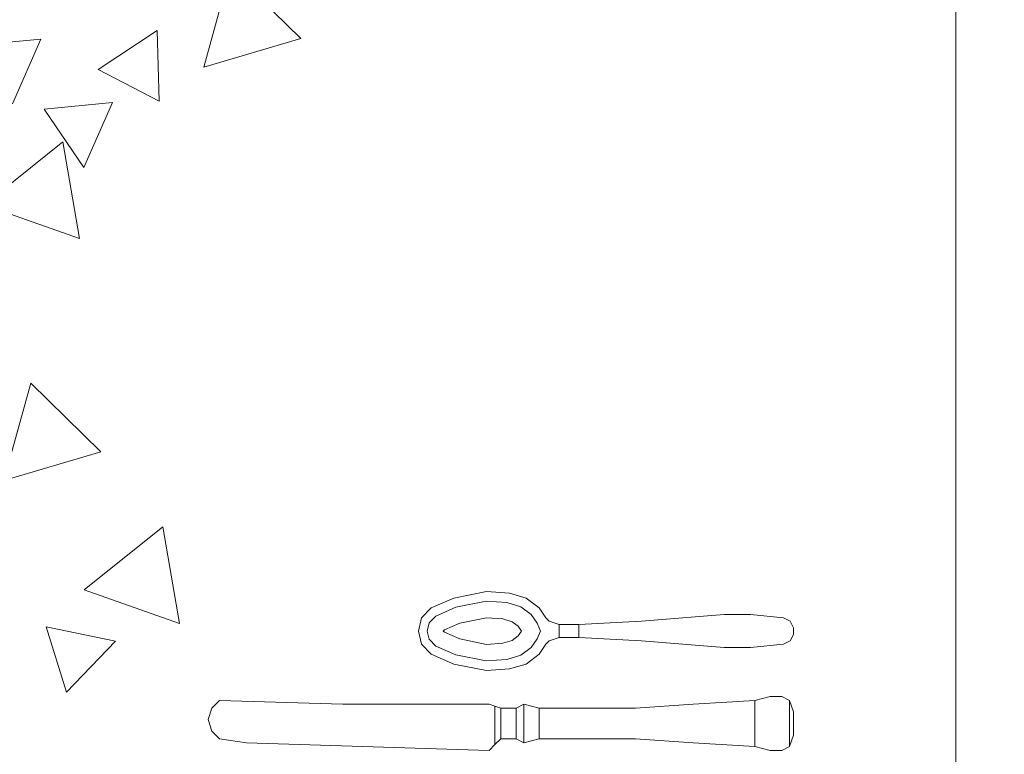
# Model space of a CAD drawing. Units: inches. Extents: x 375 to 1122, y 27 to 1069.
# Tile 114 of 155: x 731.28 to 747.02, y 874.87 to 886.61. Entities that reach past the tile are written whole.
import ezdxf

# ---------------------------------------------------------------- set-up
doc = ezdxf.new("R2010")
doc.units = ezdxf.units.IN
doc.layers.add('A-ANNO-DIMS', color=2, linetype='Continuous', lineweight=18)
doc.layers.add('Furniture', color=30, linetype='Continuous', lineweight=18)
doc.styles.get("Standard").update_dxf_attribs({"font": 'arial.ttf'})
doc.dimstyles.new('ISO-25', dxfattribs={"dimtxt": 12, "dimasz": 2.5, "dimexe": 1.5, "dimexo": 1.5, "dimtad": 1, "dimdec": 1, "dimlunit": 3, "dimtxsty": 'Standard', "dimblk": 'ARCHTICK', "dimcen": 2.5, "dimadec": 0, "dimazin": 0, "dimtfac": 1, "dimtdec": 1, "dimtmove": 0, "dimatfit": 3, "dimfxl": 1.5, "dimfxlon": 1, "dimarcsym": 0})

# ---------------------------------------------------------------- blocks, each defined once
blk = doc.blocks.new('A$C403C54AD')
for p, q in [((0.83575, 1.53256, -0.0006), (1.99923, 1.53256, -0.0006)), ((1.27287, 1.24271, -0.0006), (1.30033, 1.27073, -0.0006)), ((1.30033, 1.27073, -0.0006), (1.31179, 1.23198, -0.0006)), ((1.31179, 1.23198, -0.0006), (1.27287, 1.24271, -0.0006)), ((1.49552, 1.21567, -0.0006), (1.53418, 1.22227, -0.0006)), ((1.53418, 1.22227, -0.0006), (1.52076, 1.18416, -0.0006)), ((1.29718, 1.21338, -0.0006), (1.32543, 1.2141, -0.0006)), ((1.31273, 1.18976, -0.0006), (1.29718, 1.21338, -0.0006)), ((1.32543, 1.2141, -0.0006), (1.31273, 1.18976, -0.0006)), ((1.52076, 1.18416, -0.0006), (1.49552, 1.21567, -0.0006)), ((1.53546, 1.16895, -0.0006), (1.54117, 1.19665, -0.0006)), ((1.54117, 1.19665, -0.0006), (1.56166, 1.17718, -0.0006)), ((1.32856, 1.16813, -0.0006), (1.32599, 1.19547, -0.0006)), ((1.32599, 1.19547, -0.0006), (1.35188, 1.18409, -0.0006)), ((1.43807, 1.16281, -0.0006), (1.46553, 1.19082, -0.0006)), ((1.46553, 1.19082, -0.0006), (1.47699, 1.15208, -0.0006)), ((1.35188, 1.18409, -0.0006), (1.32856, 1.16813, -0.0006)), ((1.34169, 1.17565, -0.0006), (1.38035, 1.18225, -0.0006)), ((1.38035, 1.18225, -0.0006), (1.36693, 1.14415, -0.0006)), ((1.56166, 1.17718, -0.0006), (1.53546, 1.16895, -0.0006)), ((1.36693, 1.14415, -0.0006), (1.34169, 1.17565, -0.0006)), ((1.30057, 1.1669, -0.0006), (1.32646, 1.15553, -0.0006)), ((1.30314, 1.13957, -0.0006), (1.30057, 1.1669, -0.0006)), ((1.47699, 1.15208, -0.0006), (1.43807, 1.16281, -0.0006))]:
    blk.add_line(p, q)
for points, invisible_edges in [([(1.53323, 1.46634, -0.04237), (1.54115, 1.46634, -0.04237), (1.54247, 1.4637, -0.04257), (1.53191, 1.4637, -0.04257)], 5), ([(1.53323, 1.46634, -0.04634), (1.54115, 1.46634, -0.04634), (1.54247, 1.4637, -0.04655), (1.53191, 1.4637, -0.04655)], 5), ([(1.53851, 1.46766, -0.04251), (1.53587, 1.46766, -0.04251), (1.53323, 1.46634, -0.04237), (1.54115, 1.46634, -0.04237)], 4), ([(1.53851, 1.46766, -0.04605), (1.53587, 1.46766, -0.04605), (1.53323, 1.46634, -0.04634), (1.54115, 1.46634, -0.04634)], 4), ([(1.56336, 1.46304, -0.03581), (1.58491, 1.46304, -0.03581), (1.58337, 1.46612, -0.03734), (1.5649, 1.46612, -0.03734)], 1), ([(1.56336, 1.46304, -0.04504), (1.58491, 1.46304, -0.04504), (1.58337, 1.46612, -0.0435), (1.5649, 1.46612, -0.0435)], 1), ([(1.54247, 1.4637, -0.04257), (1.53191, 1.4637, -0.04257), (1.53059, 1.45051, -0.0426), (1.54379, 1.45051, -0.0426)], 5), ([(1.54247, 1.4637, -0.04655), (1.53191, 1.4637, -0.04655), (1.53059, 1.45051, -0.04658), (1.54379, 1.45051, -0.04658)], 5), ([(1.58491, 1.45842, -0.03427), (1.56336, 1.45842, -0.03427), (1.56336, 1.46304, -0.03581), (1.58491, 1.46304, -0.03581)], 5), ([(1.58491, 1.45842, -0.04658), (1.56336, 1.45842, -0.04658), (1.56336, 1.46304, -0.04504), (1.58491, 1.46304, -0.04504)], 5), ([(1.5649, 1.45227, -0.03581), (1.58337, 1.45227, -0.03581), (1.58491, 1.45842, -0.03427), (1.56336, 1.45842, -0.03427)], 4), ([(1.5649, 1.45227, -0.04504), (1.58337, 1.45227, -0.04504), (1.58491, 1.45842, -0.04658), (1.56336, 1.45842, -0.04658)], 4), ([(1.58183, 1.42764, -0.03427), (1.56644, 1.42764, -0.03427), (1.5649, 1.45227, -0.03581), (1.58337, 1.45227, -0.03581)], 1), ([(1.58183, 1.42764, -0.04658), (1.56644, 1.42764, -0.04658), (1.5649, 1.45227, -0.04504), (1.58337, 1.45227, -0.04504)], 1), ([(1.53059, 1.45051, -0.0426), (1.54379, 1.45051, -0.0426), (1.54379, 1.43995, -0.04232), (1.53059, 1.43995, -0.04232)], 5), ([(1.53059, 1.45051, -0.04658), (1.54379, 1.45051, -0.04658), (1.54379, 1.43995, -0.0463), (1.53059, 1.43995, -0.0463)], 5), ([(1.54379, 1.43995, -0.0463), (1.53059, 1.43995, -0.0463), (1.53323, 1.40697, -0.04292), (1.54115, 1.40697, -0.04292)], 5), ([(1.53059, 1.43995, -0.0463), (1.53059, 1.43995, -0.04232), (1.53323, 1.40697, -0.04028), (1.53323, 1.40697, -0.04292)], 4), ([(1.54379, 1.43995, -0.04232), (1.53059, 1.43995, -0.04232), (1.53323, 1.40697, -0.04028), (1.54115, 1.40697, -0.04028)], 5), ([(1.54115, 1.40697, -0.04292), (1.54115, 1.40697, -0.04028), (1.54379, 1.43995, -0.04232), (1.54379, 1.43995, -0.0463)], 1), ([(1.56797, 1.40455, -0.03427), (1.58029, 1.40455, -0.03427), (1.58183, 1.42764, -0.03427), (1.56644, 1.42764, -0.03427)], 5), ([(1.56797, 1.40455, -0.04658), (1.58029, 1.40455, -0.04658), (1.58183, 1.42764, -0.04658), (1.56644, 1.42764, -0.04658)], 5), ([(1.53323, 1.40697, -0.04028), (1.54115, 1.40697, -0.04028), (1.53983, 1.3819, -0.03779), (1.53455, 1.3819, -0.03779)], 1), ([(1.53323, 1.40697, -0.04028), (1.53323, 1.40697, -0.04292), (1.53455, 1.3819, -0.04001), (1.53455, 1.3819, -0.03779)], 5), ([(1.53323, 1.40697, -0.04292), (1.54115, 1.40697, -0.04292), (1.53983, 1.3819, -0.04001), (1.53455, 1.3819, -0.04001)], 1), ([(1.53983, 1.3819, -0.03779), (1.53983, 1.3819, -0.04001), (1.54115, 1.40697, -0.04292), (1.54115, 1.40697, -0.04028)], 5), ([(1.58029, 1.36607, -0.03581), (1.56797, 1.36607, -0.03581), (1.56797, 1.40455, -0.03427), (1.58029, 1.40455, -0.03427)], 4), ([(1.58029, 1.36607, -0.04504), (1.56797, 1.36607, -0.04504), (1.56797, 1.40455, -0.04658), (1.58029, 1.40455, -0.04658)], 4), ([(1.53455, 1.3819, -0.04001), (1.53455, 1.3819, -0.03779), (1.53455, 1.37399, -0.03842), (1.53455, 1.37399, -0.04064)], 5), ([(1.53983, 1.37399, -0.04064), (1.53983, 1.37399, -0.03842), (1.53983, 1.3819, -0.03779), (1.53983, 1.3819, -0.04001)], 5), ([(1.53455, 1.37399, -0.03842), (1.53983, 1.37399, -0.03842), (1.54115, 1.37003, -0.04027), (1.53323, 1.37003, -0.04027)], 4), ([(1.53455, 1.37399, -0.03842), (1.53455, 1.37399, -0.04064), (1.53323, 1.37003, -0.04236), (1.53323, 1.37003, -0.04027)], 5), ([(1.53455, 1.37399, -0.04064), (1.53983, 1.37399, -0.04064), (1.54115, 1.37003, -0.04236), (1.53323, 1.37003, -0.04236)], 4), ([(1.53983, 1.37399, -0.04064), (1.53983, 1.37399, -0.03842), (1.54115, 1.37003, -0.04027), (1.54115, 1.37003, -0.04236)], 5), ([(1.54115, 1.37003, -0.04027), (1.53323, 1.37003, -0.04027), (1.53191, 1.3687, -0.041), (1.54247, 1.3687, -0.041)], 5), ([(1.54115, 1.37003, -0.04236), (1.53323, 1.37003, -0.04236), (1.53191, 1.3687, -0.04315), (1.54247, 1.3687, -0.04315)], 5), ([(1.53323, 1.37003, -0.04236), (1.53323, 1.37003, -0.04027), (1.53191, 1.3687, -0.041), (1.53191, 1.3687, -0.04315)], 1), ([(1.54115, 1.37003, -0.04027), (1.54115, 1.37003, -0.04236), (1.54247, 1.3687, -0.04315), (1.54247, 1.3687, -0.041)], 1), ([(1.52796, 1.36608, -0.04195), (1.53064, 1.36289, -0.04423), (1.52749, 1.35867, -0.04406), (1.524, 1.36082, -0.04147)], 5), ([(1.52796, 1.36608, -0.04063), (1.53064, 1.36289, -0.04291), (1.52749, 1.35867, -0.04274), (1.524, 1.36082, -0.04015)], 5), ([(1.53405, 1.36518, -0.04424), (1.53191, 1.3687, -0.04315), (1.52796, 1.36608, -0.04195), (1.53064, 1.36289, -0.04423)], 5), ([(1.53405, 1.36518, -0.04292), (1.53191, 1.3687, -0.041), (1.52796, 1.36608, -0.04063), (1.53064, 1.36289, -0.04291)], 5), ([(1.53191, 1.3687, -0.04315), (1.53719, 1.3687, -0.04315), (1.53719, 1.36654, -0.04406), (1.53405, 1.36518, -0.04424)], 11), ([(1.53191, 1.3687, -0.041), (1.53719, 1.3687, -0.041), (1.53719, 1.36654, -0.04274), (1.53405, 1.36518, -0.04292)], 11), ([(1.53405, 1.36518, -0.04424), (1.53719, 1.35902, -0.04627), (1.53719, 1.35902, -0.04627), (1.53719, 1.36654, -0.04406)], 5), ([(1.53405, 1.36518, -0.04292), (1.53719, 1.35902, -0.04495), (1.53719, 1.35902, -0.04495), (1.53719, 1.36654, -0.04274)], 5), ([(1.54247, 1.3687, -0.04315), (1.53719, 1.3687, -0.04315), (1.53719, 1.36654, -0.04406), (1.54033, 1.36518, -0.04424)], 11), ([(1.54247, 1.3687, -0.041), (1.53719, 1.3687, -0.041), (1.53719, 1.36654, -0.04274), (1.54033, 1.36518, -0.04292)], 11), ([(1.54033, 1.36518, -0.04424), (1.53719, 1.35902, -0.04627), (1.53719, 1.35902, -0.04627), (1.53719, 1.36654, -0.04406)], 5), ([(1.54033, 1.36518, -0.04292), (1.53719, 1.35902, -0.04495), (1.53719, 1.35902, -0.04495), (1.53719, 1.36654, -0.04274)], 5), ([(1.54033, 1.36518, -0.04292), (1.54247, 1.3687, -0.041), (1.54643, 1.36608, -0.04063), (1.54374, 1.36289, -0.04291)], 5), ([(1.54643, 1.36608, -0.04195), (1.54374, 1.36289, -0.04423), (1.54689, 1.35867, -0.04406), (1.55038, 1.36082, -0.04147)], 5), ([(1.54643, 1.36608, -0.04063), (1.54374, 1.36289, -0.04291), (1.54689, 1.35867, -0.04274), (1.55038, 1.36082, -0.04015)], 5), ([(1.52749, 1.35867, -0.04406), (1.53346, 1.3553, -0.04638), (1.53523, 1.35767, -0.04647), (1.53064, 1.36289, -0.04423)], 5), ([(1.52749, 1.35867, -0.04274), (1.53346, 1.3553, -0.04506), (1.53523, 1.35767, -0.04515), (1.53064, 1.36289, -0.04291)], 5), ([(1.53523, 1.35767, -0.04647), (1.53064, 1.36289, -0.04423), (1.53405, 1.36518, -0.04424), (1.53719, 1.35902, -0.04627)], 5), ([(1.53523, 1.35767, -0.04515), (1.53064, 1.36289, -0.04291), (1.53405, 1.36518, -0.04292), (1.53719, 1.35902, -0.04495)], 5), ([(1.53915, 1.35767, -0.04647), (1.54374, 1.36289, -0.04423), (1.54033, 1.36518, -0.04424), (1.53719, 1.35902, -0.04627)], 5), ([(1.53915, 1.35767, -0.04515), (1.54374, 1.36289, -0.04291), (1.54033, 1.36518, -0.04292), (1.53719, 1.35902, -0.04495)], 5), ([(1.54689, 1.35867, -0.04406), (1.54092, 1.3553, -0.04638), (1.53915, 1.35767, -0.04647), (1.54374, 1.36289, -0.04423)], 5), ([(1.54689, 1.35867, -0.04274), (1.54092, 1.3553, -0.04506), (1.53915, 1.35767, -0.04515), (1.54374, 1.36289, -0.04291)], 5), ([(1.52749, 1.35867, -0.04274), (1.524, 1.36082, -0.04015), (1.52202, 1.35422, -0.03974), (1.52583, 1.35316, -0.04222)], 5), ([(1.52749, 1.35867, -0.04406), (1.524, 1.36082, -0.04147), (1.52202, 1.35422, -0.04106), (1.52583, 1.35316, -0.04354)], 5), ([(1.53234, 1.35158, -0.04614), (1.52583, 1.35316, -0.04354), (1.52749, 1.35867, -0.04406), (1.53346, 1.3553, -0.04638)], 5), ([(1.53234, 1.35158, -0.04482), (1.52583, 1.35316, -0.04222), (1.52749, 1.35867, -0.04274), (1.53346, 1.3553, -0.04506)], 5), ([(1.53523, 1.35767, -0.04647), (1.53915, 1.35767, -0.04647), (1.53719, 1.35902, -0.04627)], 1), ([(1.53523, 1.35767, -0.04515), (1.53915, 1.35767, -0.04515), (1.53719, 1.35902, -0.04495)], 1), ([(1.54204, 1.35158, -0.04482), (1.54855, 1.35316, -0.04222), (1.54689, 1.35867, -0.04274), (1.54092, 1.3553, -0.04506)], 5), ([(1.54689, 1.35867, -0.04274), (1.55038, 1.36082, -0.04015), (1.55236, 1.35422, -0.03974), (1.54855, 1.35316, -0.04222)], 5), ([(1.54689, 1.35867, -0.04406), (1.55038, 1.36082, -0.04147), (1.55236, 1.35422, -0.04106), (1.54855, 1.35316, -0.04354)], 5), ([(1.52202, 1.35422, -0.03974), (1.52583, 1.35316, -0.04222), (1.52524, 1.34491, -0.04133), (1.52136, 1.34501, -0.03888)], 5), ([(1.52202, 1.35422, -0.04106), (1.52583, 1.35316, -0.04354), (1.52524, 1.34491, -0.04265), (1.52136, 1.34501, -0.0402)], 5), ([(1.53234, 1.35158, -0.04614), (1.54204, 1.35158, -0.04614), (1.54092, 1.3553, -0.04638), (1.53346, 1.3553, -0.04638)], 5), ([(1.53234, 1.35158, -0.04482), (1.54204, 1.35158, -0.04482), (1.54092, 1.3553, -0.04506), (1.53346, 1.3553, -0.04506)], 5), ([(1.54092, 1.3553, -0.04638), (1.53346, 1.3553, -0.04638), (1.53523, 1.35767, -0.04647), (1.53915, 1.35767, -0.04647)], 5), ([(1.54092, 1.3553, -0.04506), (1.53346, 1.3553, -0.04506), (1.53523, 1.35767, -0.04515), (1.53915, 1.35767, -0.04515)], 5), ([(1.55236, 1.35422, -0.03974), (1.54855, 1.35316, -0.04222), (1.54914, 1.34491, -0.04133), (1.55302, 1.34501, -0.03888)], 5), ([(1.55236, 1.35422, -0.04106), (1.54855, 1.35316, -0.04354), (1.54914, 1.34491, -0.04265), (1.55302, 1.34501, -0.0402)], 5), ([(1.56797, 1.35684, -0.04504), (1.56797, 1.35684, -0.03581), (1.56797, 1.35068, -0.03581), (1.56797, 1.35068, -0.04504)], 4), ([(1.58029, 1.35068, -0.04504), (1.58029, 1.35068, -0.03581), (1.58029, 1.35684, -0.03581), (1.58029, 1.35684, -0.04504)], 1), ([(1.52524, 1.34491, -0.04265), (1.53187, 1.34497, -0.0452), (1.53234, 1.35158, -0.04614), (1.52583, 1.35316, -0.04354)], 5), ([(1.52524, 1.34491, -0.04133), (1.53187, 1.34497, -0.04388), (1.53234, 1.35158, -0.04482), (1.52583, 1.35316, -0.04222)], 5), ([(1.54252, 1.34497, -0.0452), (1.53187, 1.34497, -0.0452), (1.53234, 1.35158, -0.04614), (1.54204, 1.35158, -0.04614)], 5), ([(1.54252, 1.34497, -0.04388), (1.53187, 1.34497, -0.04388), (1.53234, 1.35158, -0.04482), (1.54204, 1.35158, -0.04482)], 5), ([(1.54914, 1.34491, -0.04265), (1.54252, 1.34497, -0.0452), (1.54204, 1.35158, -0.04614), (1.54855, 1.35316, -0.04354)], 5), ([(1.54914, 1.34491, -0.04133), (1.54252, 1.34497, -0.04388), (1.54204, 1.35158, -0.04482), (1.54855, 1.35316, -0.04222)], 5), ([(1.56797, 1.35068, -0.03581), (1.56797, 1.35068, -0.04504), (1.56721, 1.34837, -0.04196), (1.56721, 1.34837, -0.03888)], 5), ([(1.5826, 1.34837, -0.03888), (1.5826, 1.34837, -0.04196), (1.58029, 1.35068, -0.04504), (1.58029, 1.35068, -0.03581)], 5), ([(1.58491, 1.34606, -0.03965), (1.56644, 1.34606, -0.03965), (1.56721, 1.34837, -0.03888), (1.5826, 1.34837, -0.03888)], 1), ([(1.58491, 1.34606, -0.04119), (1.56644, 1.34606, -0.04119), (1.56721, 1.34837, -0.04196), (1.5826, 1.34837, -0.04196)], 1), ([(1.56721, 1.34837, -0.04196), (1.56721, 1.34837, -0.03888), (1.56644, 1.34606, -0.03965), (1.56644, 1.34606, -0.04119)], 5), ([(1.56644, 1.28757, -0.03965), (1.58183, 1.24909, -0.03965), (1.58491, 1.34606, -0.03965), (1.56644, 1.34606, -0.03965)], 5), ([(1.56644, 1.28757, -0.04119), (1.58183, 1.24909, -0.04119), (1.58491, 1.34606, -0.04119), (1.56644, 1.34606, -0.04119)], 5), ([(1.56644, 1.34606, -0.03965), (1.56644, 1.34606, -0.04119), (1.56644, 1.28757, -0.04119), (1.56644, 1.28757, -0.03965)], 5), ([(1.58183, 1.24909, -0.04119), (1.58183, 1.24909, -0.03965), (1.58491, 1.34606, -0.03965), (1.58491, 1.34606, -0.04119)], 5), ([(1.58491, 1.34606, -0.04119), (1.58491, 1.34606, -0.03965), (1.5826, 1.34837, -0.03888), (1.5826, 1.34837, -0.04196)], 5), ([(1.52524, 1.34491, -0.04265), (1.52136, 1.34501, -0.0402), (1.524, 1.33198, -0.03816), (1.5277, 1.33278, -0.04067)], 5), ([(1.52524, 1.34491, -0.04133), (1.52136, 1.34501, -0.03888), (1.524, 1.33198, -0.03684), (1.5277, 1.33278, -0.03935)], 5), ([(1.53402, 1.33436, -0.04216), (1.5277, 1.33278, -0.03935), (1.52524, 1.34491, -0.04133), (1.53187, 1.34497, -0.04388)], 5), ([(1.53402, 1.33436, -0.04348), (1.5277, 1.33278, -0.04067), (1.52524, 1.34491, -0.04265), (1.53187, 1.34497, -0.0452)], 5), ([(1.53402, 1.33436, -0.04216), (1.54037, 1.33436, -0.04216), (1.54252, 1.34497, -0.04388), (1.53187, 1.34497, -0.04388)], 5), ([(1.53402, 1.33436, -0.04348), (1.54037, 1.33436, -0.04348), (1.54252, 1.34497, -0.0452), (1.53187, 1.34497, -0.0452)], 5), ([(1.54037, 1.33436, -0.04216), (1.54668, 1.33278, -0.03935), (1.54914, 1.34491, -0.04133), (1.54252, 1.34497, -0.04388)], 5), ([(1.54037, 1.33436, -0.04348), (1.54668, 1.33278, -0.04067), (1.54914, 1.34491, -0.04265), (1.54252, 1.34497, -0.0452)], 5), ([(1.54914, 1.34491, -0.04265), (1.55302, 1.34501, -0.0402), (1.55038, 1.33198, -0.03816), (1.54668, 1.33278, -0.04067)], 5), ([(1.54914, 1.34491, -0.04133), (1.55302, 1.34501, -0.03888), (1.55038, 1.33198, -0.03684), (1.54668, 1.33278, -0.03935)], 5), ([(1.53121, 1.32476, -0.03896), (1.53675, 1.32814, -0.04186), (1.53402, 1.33436, -0.04348), (1.5277, 1.33278, -0.04067)], 5), ([(1.53121, 1.32476, -0.03764), (1.53675, 1.32814, -0.04054), (1.53402, 1.33436, -0.04216), (1.5277, 1.33278, -0.03935)], 5), ([(1.53763, 1.32814, -0.04186), (1.53675, 1.32814, -0.04186), (1.53402, 1.33436, -0.04348), (1.54037, 1.33436, -0.04348)], 5), ([(1.53763, 1.32814, -0.04054), (1.53675, 1.32814, -0.04054), (1.53402, 1.33436, -0.04216), (1.54037, 1.33436, -0.04216)], 5), ([(1.54318, 1.32476, -0.03896), (1.53763, 1.32814, -0.04186), (1.54037, 1.33436, -0.04348), (1.54668, 1.33278, -0.04067)], 5), ([(1.54318, 1.32476, -0.03764), (1.53763, 1.32814, -0.04054), (1.54037, 1.33436, -0.04216), (1.54668, 1.33278, -0.03935)], 5), ([(1.524, 1.33198, -0.03816), (1.5277, 1.33278, -0.04067), (1.53121, 1.32476, -0.03896), (1.52796, 1.32291, -0.03632)], 5), ([(1.524, 1.33198, -0.03684), (1.5277, 1.33278, -0.03935), (1.53121, 1.32476, -0.03764), (1.52796, 1.32291, -0.035)], 5), ([(1.55038, 1.33198, -0.03816), (1.54668, 1.33278, -0.04067), (1.54318, 1.32476, -0.03896), (1.54643, 1.32291, -0.03632)], 5), ([(1.55038, 1.33198, -0.03684), (1.54668, 1.33278, -0.03935), (1.54318, 1.32476, -0.03764), (1.54643, 1.32291, -0.035)], 5), ([(1.53675, 1.32814, -0.04054), (1.53388, 1.32213, -0.03709), (1.53121, 1.32476, -0.03764), (1.53675, 1.32814, -0.04054)], 5), ([(1.53675, 1.32814, -0.04186), (1.53388, 1.32213, -0.03841), (1.53121, 1.32476, -0.03896), (1.53675, 1.32814, -0.04186)], 5), ([(1.53719, 1.32132, -0.0369), (1.53719, 1.32772, -0.0404), (1.53675, 1.32814, -0.04054), (1.53388, 1.32213, -0.03709)], 5), ([(1.53719, 1.32132, -0.03822), (1.53719, 1.32772, -0.04172), (1.53675, 1.32814, -0.04186), (1.53388, 1.32213, -0.03841)], 5), ([(1.53719, 1.32772, -0.0404), (1.53675, 1.32814, -0.04054), (1.53763, 1.32814, -0.04054), (1.53719, 1.32772, -0.0404)], 2), ([(1.53719, 1.32772, -0.04172), (1.53675, 1.32814, -0.04186), (1.53763, 1.32814, -0.04186), (1.53719, 1.32772, -0.04172)], 2), ([(1.53719, 1.32132, -0.0369), (1.53719, 1.32772, -0.0404), (1.53763, 1.32814, -0.04054), (1.5405, 1.32213, -0.03709)], 5), ([(1.53719, 1.32132, -0.03822), (1.53719, 1.32772, -0.04172), (1.53763, 1.32814, -0.04186), (1.5405, 1.32213, -0.03841)], 5), ([(1.53763, 1.32814, -0.04054), (1.5405, 1.32213, -0.03709), (1.54318, 1.32476, -0.03764), (1.53763, 1.32814, -0.04054)], 5), ([(1.53763, 1.32814, -0.04186), (1.5405, 1.32213, -0.03841), (1.54318, 1.32476, -0.03896), (1.53763, 1.32814, -0.04186)], 5), ([(1.53121, 1.32476, -0.03896), (1.52796, 1.32291, -0.03632), (1.53191, 1.31907, -0.03523), (1.53388, 1.32213, -0.03841)], 5), ([(1.53121, 1.32476, -0.03764), (1.52796, 1.32291, -0.035), (1.53191, 1.31907, -0.03391), (1.53388, 1.32213, -0.03709)], 5), ([(1.54318, 1.32476, -0.03896), (1.54643, 1.32291, -0.03632), (1.54247, 1.31907, -0.03523), (1.5405, 1.32213, -0.03841)], 5), ([(1.54318, 1.32476, -0.03764), (1.54643, 1.32291, -0.035), (1.54247, 1.31907, -0.03391), (1.5405, 1.32213, -0.03709)], 5), ([(1.53191, 1.31907, -0.03523), (1.53388, 1.32213, -0.03841), (1.53719, 1.32132, -0.03822), (1.53719, 1.31776, -0.03505)], 5), ([(1.53191, 1.31907, -0.03391), (1.53388, 1.32213, -0.03709), (1.53719, 1.32132, -0.0369), (1.53719, 1.31776, -0.03373)], 5), ([(1.54247, 1.31907, -0.03523), (1.5405, 1.32213, -0.03841), (1.53719, 1.32132, -0.03822), (1.53719, 1.31776, -0.03505)], 5), ([(1.54247, 1.31907, -0.03391), (1.5405, 1.32213, -0.03709), (1.53719, 1.32132, -0.0369), (1.53719, 1.31776, -0.03373)], 5), ([(1.58029, 1.23832, -0.03965), (1.5649, 1.23832, -0.03965), (1.56644, 1.28757, -0.03965), (1.58183, 1.24909, -0.03965)], 5), ([(1.58029, 1.23832, -0.04119), (1.5649, 1.23832, -0.04119), (1.56644, 1.28757, -0.04119), (1.58183, 1.24909, -0.04119)], 5), ([(1.56644, 1.28757, -0.04119), (1.56644, 1.28757, -0.03965), (1.5649, 1.23832, -0.03965), (1.5649, 1.23832, -0.04119)], 5), ([(1.58029, 1.23832, -0.03965), (1.58029, 1.23832, -0.04119), (1.58183, 1.24909, -0.04119), (1.58183, 1.24909, -0.03965)], 5), ([(1.56797, 1.23524, -0.03965), (1.57721, 1.23524, -0.03965), (1.58029, 1.23832, -0.03965), (1.5649, 1.23832, -0.03965)], 5), ([(1.56797, 1.23524, -0.04119), (1.57721, 1.23524, -0.04119), (1.58029, 1.23832, -0.04119), (1.5649, 1.23832, -0.04119)], 5), ([(1.5649, 1.23832, -0.03965), (1.5649, 1.23832, -0.04119), (1.56797, 1.23524, -0.04119), (1.56797, 1.23524, -0.03965)], 5), ([(1.57721, 1.23524, -0.04119), (1.57721, 1.23524, -0.03965), (1.58029, 1.23832, -0.03965), (1.58029, 1.23832, -0.04119)], 5), ([(1.57259, 1.2337, -0.03965), (1.57259, 1.2337, -0.03965), (1.56797, 1.23524, -0.03965), (1.57721, 1.23524, -0.03965)], 4), ([(1.57259, 1.2337, -0.04119), (1.57259, 1.2337, -0.04119), (1.56797, 1.23524, -0.04119), (1.57721, 1.23524, -0.04119)], 4), ([(1.56797, 1.23524, -0.04119), (1.56797, 1.23524, -0.03965), (1.57259, 1.2337, -0.03965), (1.57259, 1.2337, -0.04119)], 1), ([(1.57259, 1.2337, -0.03965), (1.57259, 1.2337, -0.04119), (1.57721, 1.23524, -0.04119), (1.57721, 1.23524, -0.03965)], 4)]:
    blk.add_3dface(points, dxfattribs=dict(invisible_edges=invisible_edges))
for points in [[(1.53323, 1.46634, -0.04237), (1.53323, 1.46634, -0.04634), (1.53191, 1.4637, -0.04655), (1.53191, 1.4637, -0.04257)], [(1.53587, 1.46766, -0.04605), (1.53587, 1.46766, -0.04251), (1.53323, 1.46634, -0.04237), (1.53323, 1.46634, -0.04634)], [(1.53851, 1.46766, -0.04251), (1.53851, 1.46766, -0.04605), (1.53587, 1.46766, -0.04605), (1.53587, 1.46766, -0.04251)], [(1.54115, 1.46634, -0.04634), (1.54115, 1.46634, -0.04237), (1.53851, 1.46766, -0.04251), (1.53851, 1.46766, -0.04605)], [(1.54247, 1.4637, -0.04257), (1.54247, 1.4637, -0.04655), (1.54115, 1.46634, -0.04634), (1.54115, 1.46634, -0.04237)], [(1.5649, 1.46612, -0.03734), (1.5649, 1.46612, -0.0435), (1.56336, 1.46304, -0.04504), (1.56336, 1.46304, -0.03581)], [(1.58337, 1.46612, -0.03734), (1.5649, 1.46612, -0.03734), (1.56951, 1.46766, -0.04042), (1.57875, 1.46766, -0.04042)], [(1.56951, 1.46766, -0.04042), (1.56951, 1.46766, -0.04042), (1.5649, 1.46612, -0.03734), (1.5649, 1.46612, -0.0435)], [(1.58337, 1.46612, -0.0435), (1.5649, 1.46612, -0.0435), (1.56951, 1.46766, -0.04042), (1.57875, 1.46766, -0.04042)], [(1.58337, 1.46612, -0.03734), (1.58337, 1.46612, -0.0435), (1.57875, 1.46766, -0.04042)], [(1.58491, 1.46304, -0.04504), (1.58491, 1.46304, -0.03581), (1.58337, 1.46612, -0.03734), (1.58337, 1.46612, -0.0435)], [(1.53191, 1.4637, -0.04655), (1.53191, 1.4637, -0.04257), (1.53059, 1.45051, -0.0426), (1.53059, 1.45051, -0.04658)], [(1.54379, 1.45051, -0.04658), (1.54379, 1.45051, -0.0426), (1.54247, 1.4637, -0.04257), (1.54247, 1.4637, -0.04655)], [(1.56336, 1.46304, -0.03581), (1.56336, 1.46304, -0.04504), (1.56336, 1.45842, -0.04658), (1.56336, 1.45842, -0.03427)], [(1.58491, 1.45842, -0.03427), (1.58491, 1.45842, -0.04658), (1.58491, 1.46304, -0.04504), (1.58491, 1.46304, -0.03581)], [(1.56336, 1.45842, -0.04658), (1.56336, 1.45842, -0.03427), (1.5649, 1.45227, -0.03581), (1.5649, 1.45227, -0.04504)], [(1.58337, 1.45227, -0.04504), (1.58337, 1.45227, -0.03581), (1.58491, 1.45842, -0.03427), (1.58491, 1.45842, -0.04658)], [(1.5649, 1.45227, -0.03581), (1.5649, 1.45227, -0.04504), (1.56644, 1.42764, -0.04658), (1.56644, 1.42764, -0.03427)], [(1.58183, 1.42764, -0.03427), (1.58183, 1.42764, -0.04658), (1.58337, 1.45227, -0.04504), (1.58337, 1.45227, -0.03581)], [(1.53059, 1.45051, -0.0426), (1.53059, 1.45051, -0.04658), (1.53059, 1.43995, -0.0463), (1.53059, 1.43995, -0.04232)], [(1.54379, 1.43995, -0.04232), (1.54379, 1.43995, -0.0463), (1.54379, 1.45051, -0.04658), (1.54379, 1.45051, -0.0426)], [(1.56644, 1.42764, -0.04658), (1.56644, 1.42764, -0.03427), (1.56797, 1.40455, -0.03427), (1.56797, 1.40455, -0.04658)], [(1.58029, 1.40455, -0.04658), (1.58029, 1.40455, -0.03427), (1.58183, 1.42764, -0.03427), (1.58183, 1.42764, -0.04658)], [(1.56797, 1.40455, -0.03427), (1.56797, 1.40455, -0.04658), (1.56797, 1.36607, -0.04504), (1.56797, 1.36607, -0.03581)], [(1.58029, 1.36607, -0.03581), (1.58029, 1.36607, -0.04504), (1.58029, 1.40455, -0.04658), (1.58029, 1.40455, -0.03427)], [(1.53983, 1.3819, -0.04001), (1.53455, 1.3819, -0.04001), (1.53455, 1.37399, -0.04064), (1.53983, 1.37399, -0.04064)], [(1.53983, 1.3819, -0.03779), (1.53455, 1.3819, -0.03779), (1.53455, 1.37399, -0.03842), (1.53983, 1.37399, -0.03842)], [(1.52796, 1.36608, -0.04063), (1.52796, 1.36608, -0.04195), (1.524, 1.36082, -0.04147), (1.524, 1.36082, -0.04015)], [(1.53191, 1.3687, -0.04315), (1.53191, 1.3687, -0.041), (1.52796, 1.36608, -0.04063), (1.52796, 1.36608, -0.04195)], [(1.54643, 1.36608, -0.04195), (1.54643, 1.36608, -0.04063), (1.54247, 1.3687, -0.041), (1.54247, 1.3687, -0.04315)], [(1.55038, 1.36082, -0.04015), (1.55038, 1.36082, -0.04147), (1.54643, 1.36608, -0.04195), (1.54643, 1.36608, -0.04063)], [(1.56644, 1.35991, -0.03427), (1.58183, 1.35991, -0.03427), (1.58029, 1.36607, -0.03581), (1.56797, 1.36607, -0.03581)], [(1.56644, 1.35991, -0.04658), (1.58183, 1.35991, -0.04658), (1.58029, 1.36607, -0.04504), (1.56797, 1.36607, -0.04504)], [(1.56797, 1.36607, -0.04504), (1.56797, 1.36607, -0.03581), (1.56644, 1.35991, -0.03427), (1.56644, 1.35991, -0.04658)], [(1.58183, 1.35991, -0.04658), (1.58183, 1.35991, -0.03427), (1.58029, 1.36607, -0.03581), (1.58029, 1.36607, -0.04504)], [(1.524, 1.36082, -0.04147), (1.524, 1.36082, -0.04015), (1.52202, 1.35422, -0.03974), (1.52202, 1.35422, -0.04106)], [(1.55236, 1.35422, -0.04106), (1.55236, 1.35422, -0.03974), (1.55038, 1.36082, -0.04015), (1.55038, 1.36082, -0.04147)], [(1.58029, 1.35684, -0.03581), (1.56797, 1.35684, -0.03581), (1.56644, 1.35991, -0.03427), (1.58183, 1.35991, -0.03427)], [(1.58029, 1.35684, -0.04504), (1.56797, 1.35684, -0.04504), (1.56644, 1.35991, -0.04658), (1.58183, 1.35991, -0.04658)], [(1.56644, 1.35991, -0.03427), (1.56644, 1.35991, -0.04658), (1.56797, 1.35684, -0.04504), (1.56797, 1.35684, -0.03581)], [(1.58029, 1.35684, -0.03581), (1.58029, 1.35684, -0.04504), (1.58183, 1.35991, -0.04658), (1.58183, 1.35991, -0.03427)], [(1.52202, 1.35422, -0.03974), (1.52202, 1.35422, -0.04106), (1.52136, 1.34501, -0.0402), (1.52136, 1.34501, -0.03888)], [(1.55302, 1.34501, -0.0402), (1.55302, 1.34501, -0.03888), (1.55236, 1.35422, -0.03974), (1.55236, 1.35422, -0.04106)], [(1.56797, 1.35068, -0.03581), (1.58029, 1.35068, -0.03581), (1.58029, 1.35684, -0.03581), (1.56797, 1.35684, -0.03581)], [(1.56797, 1.35068, -0.04504), (1.58029, 1.35068, -0.04504), (1.58029, 1.35684, -0.04504), (1.56797, 1.35684, -0.04504)], [(1.5826, 1.34837, -0.03888), (1.56721, 1.34837, -0.03888), (1.56797, 1.35068, -0.03581), (1.58029, 1.35068, -0.03581)], [(1.5826, 1.34837, -0.04196), (1.56721, 1.34837, -0.04196), (1.56797, 1.35068, -0.04504), (1.58029, 1.35068, -0.04504)], [(1.52136, 1.34501, -0.0402), (1.52136, 1.34501, -0.03888), (1.524, 1.33198, -0.03684), (1.524, 1.33198, -0.03816)], [(1.55038, 1.33198, -0.03684), (1.55038, 1.33198, -0.03816), (1.55302, 1.34501, -0.0402), (1.55302, 1.34501, -0.03888)], [(1.524, 1.33198, -0.03684), (1.524, 1.33198, -0.03816), (1.52796, 1.32291, -0.03632), (1.52796, 1.32291, -0.035)], [(1.54643, 1.32291, -0.03632), (1.54643, 1.32291, -0.035), (1.55038, 1.33198, -0.03684), (1.55038, 1.33198, -0.03816)], [(1.52796, 1.32291, -0.03632), (1.52796, 1.32291, -0.035), (1.53191, 1.31907, -0.03391), (1.53191, 1.31907, -0.03523)], [(1.54247, 1.31907, -0.03391), (1.54247, 1.31907, -0.03523), (1.54643, 1.32291, -0.03632), (1.54643, 1.32291, -0.035)], [(1.53191, 1.31907, -0.03391), (1.53191, 1.31907, -0.03523), (1.53719, 1.31776, -0.03505), (1.53719, 1.31776, -0.03373)], [(1.53719, 1.31776, -0.03505), (1.53719, 1.31776, -0.03373), (1.54247, 1.31907, -0.03391), (1.54247, 1.31907, -0.03523)]]:
    blk.add_3dface(points)
blk = doc.blocks.new('_ArchTick')
at = {"color": 0, "linetype": 'ByBlock', "const_width": 0.15}
blk.add_lwpolyline([(-0.5, -0.5), (0.5, 0.5)], dxfattribs=at)
blk = doc.blocks.new('*D88')
at = {"layer": 'A-ANNO-DIMS', "color": 0, "lineweight": -2, "transparency": 16777216}
for p, q in [((731.007, 1052.528), (731.007, 1055.528)), ((854.007, 1052.528), (854.007, 1055.528)), ((731.007, 1054.028), (854.007, 1054.028))]:
    blk.add_line(p, q, dxfattribs=at)
at = {"layer": 'Defpoints', "color": 0, "transparency": 16777216}
for p in [(854.007, 1054.028), (731.007, 502.528), (854.007, 502.528)]:
    blk.add_point(p, dxfattribs=at)
at = {"layer": 'A-ANNO-DIMS', "color": 0, "lineweight": -2, "transparency": 16777216, "xscale": 2.5, "yscale": 2.5, "zscale": 2.5, "rotation": 180}
blk.add_blockref('_ArchTick', (731.007, 1054.028), dxfattribs=at)
at = {"layer": 'A-ANNO-DIMS', "color": 0, "lineweight": -2, "transparency": 16777216, "xscale": 2.5, "yscale": 2.5, "zscale": 2.5}
blk.add_blockref('_ArchTick', (854.007, 1054.028), dxfattribs=at)
at = {"layer": 'A-ANNO-DIMS', "color": 0, "transparency": 16777216, "insert": (792.507, 1060.784), "char_height": 12, "attachment_point": 5}
blk.add_mtext('10\'-3"', dxfattribs=at)
blk = doc.blocks.new('*D91')
at = {"layer": 'A-ANNO-DIMS', "color": 0, "lineweight": -2, "transparency": 16777216}
for p, q in [((728.007, 1052.528), (728.007, 1055.528)), ((788.007, 1052.528), (788.007, 1055.528)), ((728.007, 1054.028), (788.007, 1054.028))]:
    blk.add_line(p, q, dxfattribs=at)
at = {"layer": 'Defpoints', "color": 0, "transparency": 16777216}
for p in [(788.007, 1054.028), (728.007, 774.028), (788.007, 774.028)]:
    blk.add_point(p, dxfattribs=at)
at = {"layer": 'A-ANNO-DIMS', "color": 0, "lineweight": -2, "transparency": 16777216, "xscale": 2.5, "yscale": 2.5, "zscale": 2.5, "rotation": 180}
blk.add_blockref('_ArchTick', (728.007, 1054.028), dxfattribs=at)
at = {"layer": 'A-ANNO-DIMS', "color": 0, "lineweight": -2, "transparency": 16777216, "xscale": 2.5, "yscale": 2.5, "zscale": 2.5}
blk.add_blockref('_ArchTick', (788.007, 1054.028), dxfattribs=at)
at = {"layer": 'A-ANNO-DIMS', "color": 0, "transparency": 16777216, "insert": (758.007, 1060.78), "char_height": 12, "attachment_point": 5}
blk.add_mtext('5\'-0"', dxfattribs=at)

msp = doc.modelspace()

# ---------------------------------------------------------------- block references
at = {"layer": 'Furniture', "xscale": 39.9918517141215, "yscale": 39.9918517141215, "zscale": 39.9918517141215, "rotation": 270}
msp.add_blockref('A$C403C54AD', (684.955, 938.316, 0.024), dxfattribs=at)

# ---------------------------------------------------------------- dimensions: what is measured, and where the dimension line sits
at = {"layer": 'A-ANNO-DIMS'}
for base, p1, p2, picture, middle in [((788.007, 1054.028), (728.007, 774.028), (788.007, 774.028), '*D91', (758.007, 1060.78)), ((854.007, 1054.028), (731.007, 502.528), (854.007, 502.528), '*D88', (792.507, 1060.784))]:
    dim = msp.add_linear_dim(base=base, p1=p1, p2=p2, dimstyle='ISO-25', override={"dimdec": 1, "dimlfac": 1, "dimrnd": 0, "dimzin": 1, "dimdsep": 46, "dimlunit": 4, "dimfrac": 2}, dxfattribs=at)
    dim.commit()
    dim.dimension.update_dxf_attribs({"geometry": picture, "text_midpoint": middle})

doc.saveas('drawing.dxf')
